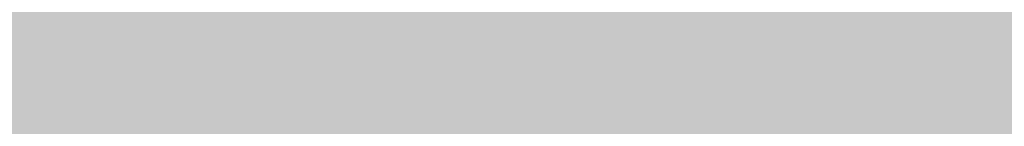
# Model space of a CAD drawing. Units: millimetres. Extents: x -22994 to 29398, y -19990 to 20176.
# Tile 77 of 135: x 226.355 to 227.437, y 84.615 to 84.732. Entities that reach past the tile are written whole.
import ezdxf
from ezdxf import colors
from ezdxf.entities.mleader import LeaderData, LeaderLine
from ezdxf.math import Vec2, Vec3

# ---------------------------------------------------------------- set-up
doc = ezdxf.new("R2010")
doc.units = ezdxf.units.MM
doc.header["$MEASUREMENT"] = 0
doc.layers.add('M-ANNO-TEXT', color=7, linetype='Continuous', lineweight=25)
doc.layers.add('M-DIMS', color=2, linetype='Continuous', lineweight=18)
doc.styles.get("Standard").update_dxf_attribs({"font": 'arial.ttf'})
doc.dimstyles.get("Standard").update_dxf_attribs({"dimtxt": 0.18, "dimasz": 10000, "dimexe": 0.18, "dimexo": 0.0625, "dimgap": 0.09, "dimtad": 0, "dimtih": 1, "dimtoh": 1, "dimdec": 0, "dimzin": 0, "dimdsep": 46, "dimtxsty": 'Standard', "dimcen": 0.09, "dimadec": 0, "dimazin": 0, "dimtfac": 1, "dimtdec": 0, "dimtofl": 0, "dimtmove": 0, "dimatfit": 3, "dimfxl": 1, "dimtolj": 1, "dimtzin": 0, "dimlwd": 30, "dimarcsym": 0})

# ---------------------------------------------------------------- blocks, each defined once
blk = doc.blocks.new('*D2')
at = {"layer": 'Defpoints', "color": 0, "transparency": 16777216}
for p in [(6.6773, 10.2713), (290.852, 10.2713), (290.852, -5.0787)]:
    blk.add_point(p, dxfattribs=at)
at = {"layer": 'M-DIMS', "color": 0, "lineweight": -2, "transparency": 16777216}
for p, q in [((6.6773, 10.2088), (6.6773, -5.2587)), ((290.852, 10.2088), (290.852, -5.2587))]:
    blk.add_line(p, q, dxfattribs=at)
at = {"layer": 'M-DIMS', "color": 0, "lineweight": 30, "transparency": 16777216}
for p, q in [((-9993.3227, -5.0787), (-19993.3227, -5.0787)), ((10290.852, -5.0787), (20290.852, -5.0787))]:
    blk.add_line(p, q, dxfattribs=at)
at = {"layer": 'M-DIMS', "color": 0, "transparency": 16777216}
for points in [[(-9993.3227, 1661.5879), (-9993.3227, -1671.7454), (6.6773, -5.0787)], [(10290.852, 1661.5879), (10290.852, -1671.7454), (290.852, -5.0787)]]:
    blk.add_solid(points, dxfattribs=at)
at = {"layer": 'M-DIMS', "color": 0, "transparency": 16777216, "insert": (148.7647, -5.0787), "char_height": 0.18, "attachment_point": 5}
blk.add_mtext('\\A1;284.2', dxfattribs=at)
blk = doc.blocks.new('*D3')
at = {"layer": 'Defpoints', "color": 0, "transparency": 16777216}
for p in [(110.2647, 204.1654), (110.2647, 176.3662), (95.8327, 127.967)]:
    blk.add_point(p, dxfattribs=at)
at = {"layer": 'M-DIMS', "color": 0, "lineweight": -2, "transparency": 16777216}
for p, q in [((95.8327, 128.0295), (95.8327, 204.3454)), ((110.2647, 176.4287), (110.2647, 204.3454))]:
    blk.add_line(p, q, dxfattribs=at)
at = {"layer": 'M-DIMS', "color": 0, "lineweight": 30, "transparency": 16777216}
for p, q in [((-9904.1673, 204.1654), (-19904.1673, 204.1654)), ((10110.2647, 204.1654), (20110.2647, 204.1654))]:
    blk.add_line(p, q, dxfattribs=at)
at = {"layer": 'M-DIMS', "color": 0, "transparency": 16777216}
for points in [[(-9904.1673, 1870.8321), (-9904.1673, -1462.5013), (95.8327, 204.1654)], [(10110.2647, 1870.8321), (10110.2647, -1462.5013), (110.2647, 204.1654)]]:
    blk.add_solid(points, dxfattribs=at)
at = {"layer": 'M-DIMS', "color": 0, "transparency": 16777216, "insert": (103.0487, 204.1654), "char_height": 0.18, "attachment_point": 5}
blk.add_mtext('\\A1;14.432', dxfattribs=at)
blk = doc.blocks.new('*D4')
at = {"layer": 'Defpoints', "color": 0, "transparency": 16777216}
for p in [(116.2647, 204.1654), (110.2647, 176.3662), (116.2647, 176.3662)]:
    blk.add_point(p, dxfattribs=at)
at = {"layer": 'M-DIMS', "color": 0, "lineweight": -2, "transparency": 16777216}
for p, q in [((110.2647, 176.4287), (110.2647, 204.3454)), ((116.2647, 176.4287), (116.2647, 204.3454))]:
    blk.add_line(p, q, dxfattribs=at)
at = {"layer": 'M-DIMS', "color": 0, "lineweight": 30, "transparency": 16777216}
for p, q in [((-9889.7353, 204.1654), (-19889.7353, 204.1654)), ((10116.2647, 204.1654), (20116.2647, 204.1654))]:
    blk.add_line(p, q, dxfattribs=at)
at = {"layer": 'M-DIMS', "color": 0, "transparency": 16777216}
for points in [[(-9889.7353, 1870.8321), (-9889.7353, -1462.5013), (110.2647, 204.1654)], [(10116.2647, 1870.8321), (10116.2647, -1462.5013), (116.2647, 204.1654)]]:
    blk.add_solid(points, dxfattribs=at)
at = {"layer": 'M-DIMS', "color": 0, "transparency": 16777216, "insert": (113.2647, 204.1654), "char_height": 0.18, "attachment_point": 5}
blk.add_mtext('\\A1;6', dxfattribs=at)
blk = doc.blocks.new('*D5')
at = {"layer": 'Defpoints', "color": 0, "transparency": 16777216}
for p in [(181.2647, 204.1654), (116.2647, 176.3662), (181.2647, 176.3662)]:
    blk.add_point(p, dxfattribs=at)
at = {"layer": 'M-DIMS', "color": 0, "lineweight": -2, "transparency": 16777216}
for p, q in [((116.2647, 176.4287), (116.2647, 204.3454)), ((181.2647, 176.4287), (181.2647, 204.3454))]:
    blk.add_line(p, q, dxfattribs=at)
at = {"layer": 'M-DIMS', "color": 0, "lineweight": 30, "transparency": 16777216}
for p, q in [((-9883.7353, 204.1654), (-19883.7353, 204.1654)), ((10181.2647, 204.1654), (20181.2647, 204.1654))]:
    blk.add_line(p, q, dxfattribs=at)
at = {"layer": 'M-DIMS', "color": 0, "transparency": 16777216}
for points in [[(-9883.7353, 1870.8321), (-9883.7353, -1462.5013), (116.2647, 204.1654)], [(10181.2647, 1870.8321), (10181.2647, -1462.5013), (181.2647, 204.1654)]]:
    blk.add_solid(points, dxfattribs=at)
at = {"layer": 'M-DIMS', "color": 0, "transparency": 16777216, "insert": (148.7647, 204.1654), "char_height": 0.18, "attachment_point": 5}
blk.add_mtext('\\A1;65', dxfattribs=at)
blk = doc.blocks.new('*D6')
at = {"layer": 'Defpoints', "color": 0, "transparency": 16777216}
for p in [(187.2647, 204.1654), (181.2647, 176.3662), (187.2647, 176.3662)]:
    blk.add_point(p, dxfattribs=at)
at = {"layer": 'M-DIMS', "color": 0, "lineweight": -2, "transparency": 16777216}
for p, q in [((181.2647, 176.4287), (181.2647, 204.3454)), ((187.2647, 176.4287), (187.2647, 204.3454))]:
    blk.add_line(p, q, dxfattribs=at)
at = {"layer": 'M-DIMS', "color": 0, "lineweight": 30, "transparency": 16777216}
for p, q in [((-9818.7353, 204.1654), (-19818.7353, 204.1654)), ((10187.2647, 204.1654), (20187.2647, 204.1654))]:
    blk.add_line(p, q, dxfattribs=at)
at = {"layer": 'M-DIMS', "color": 0, "transparency": 16777216}
for points in [[(-9818.7353, 1870.8321), (-9818.7353, -1462.5013), (181.2647, 204.1654)], [(10187.2647, 1870.8321), (10187.2647, -1462.5013), (187.2647, 204.1654)]]:
    blk.add_solid(points, dxfattribs=at)
at = {"layer": 'M-DIMS', "color": 0, "transparency": 16777216, "insert": (184.2647, 204.1654), "char_height": 0.18, "attachment_point": 5}
blk.add_mtext('\\A1;6', dxfattribs=at)
blk = doc.blocks.new('*D7')
at = {"layer": 'Defpoints', "color": 0, "transparency": 16777216}
for p in [(201.6967, 204.1654), (187.2647, 176.3662), (201.6967, 127.967)]:
    blk.add_point(p, dxfattribs=at)
at = {"layer": 'M-DIMS', "color": 0, "lineweight": -2, "transparency": 16777216}
for p, q in [((187.2647, 176.4287), (187.2647, 204.3454)), ((201.6967, 128.0295), (201.6967, 204.3454))]:
    blk.add_line(p, q, dxfattribs=at)
at = {"layer": 'M-DIMS', "color": 0, "lineweight": 30, "transparency": 16777216}
for p, q in [((-9812.7353, 204.1654), (-19812.7353, 204.1654)), ((10201.6967, 204.1654), (20201.6967, 204.1654))]:
    blk.add_line(p, q, dxfattribs=at)
at = {"layer": 'M-DIMS', "color": 0, "transparency": 16777216}
for points in [[(-9812.7353, 1870.8321), (-9812.7353, -1462.5013), (187.2647, 204.1654)], [(10201.6967, 1870.8321), (10201.6967, -1462.5013), (201.6967, 204.1654)]]:
    blk.add_solid(points, dxfattribs=at)
at = {"layer": 'M-DIMS', "color": 0, "transparency": 16777216, "insert": (194.4807, 204.1654), "char_height": 0.18, "attachment_point": 5}
blk.add_mtext('\\A1;14.432', dxfattribs=at)
blk = doc.blocks.new('*D8')
at = {"layer": 'Defpoints', "color": 0, "transparency": 16777216}
for p in [(227.6485, 204.1654), (227.6485, 146.7296), (201.6967, 127.967)]:
    blk.add_point(p, dxfattribs=at)
at = {"layer": 'M-DIMS', "color": 0, "lineweight": -2, "transparency": 16777216}
for p, q in [((201.6967, 128.0295), (201.6967, 204.3454)), ((227.6485, 146.7921), (227.6485, 204.3454))]:
    blk.add_line(p, q, dxfattribs=at)
at = {"layer": 'M-DIMS', "color": 0, "lineweight": 30, "transparency": 16777216}
for p, q in [((-9798.3033, 204.1654), (-19798.3033, 204.1654)), ((10227.6485, 204.1654), (20227.6485, 204.1654))]:
    blk.add_line(p, q, dxfattribs=at)
at = {"layer": 'M-DIMS', "color": 0, "transparency": 16777216}
for points in [[(-9798.3033, 1870.8321), (-9798.3033, -1462.5013), (201.6967, 204.1654)], [(10227.6485, 1870.8321), (10227.6485, -1462.5013), (227.6485, 204.1654)]]:
    blk.add_solid(points, dxfattribs=at)
at = {"layer": 'M-DIMS', "color": 0, "transparency": 16777216, "insert": (214.6726, 204.1654), "char_height": 0.18, "attachment_point": 5}
blk.add_mtext('\\A1;25.95', dxfattribs=at)
blk = doc.blocks.new('*D9')
at = {"layer": 'Defpoints', "color": 0, "transparency": 16777216}
for p in [(187.2647, 176.3662), (306.202, 176.3662), (290.852, 10.2713)]:
    blk.add_point(p, dxfattribs=at)
at = {"layer": 'M-DIMS', "color": 0, "lineweight": 30, "transparency": 16777216}
for p, q in [((306.202, 10176.3662), (306.202, 20176.3662)), ((306.202, -9989.7287), (306.202, -19989.7287))]:
    blk.add_line(p, q, dxfattribs=at)
at = {"layer": 'M-DIMS', "color": 0, "lineweight": -2, "transparency": 16777216}
for p, q in [((187.3272, 176.3662), (306.382, 176.3662)), ((290.9145, 10.2713), (306.382, 10.2713))]:
    blk.add_line(p, q, dxfattribs=at)
at = {"layer": 'M-DIMS', "color": 0, "transparency": 16777216}
for points in [[(-1360.4646, 10176.3662), (1972.8687, 10176.3662), (306.202, 176.3662)], [(-1360.4646, -9989.7287), (1972.8687, -9989.7287), (306.202, 10.2713)]]:
    blk.add_solid(points, dxfattribs=at)
at = {"layer": 'M-DIMS', "color": 0, "transparency": 16777216, "insert": (306.202, 93.3187), "char_height": 0.18, "attachment_point": 5}
blk.add_mtext('\\A1;166.1', dxfattribs=at)
blk = doc.blocks.new('*D10')
at = {"layer": 'Defpoints', "color": 0, "transparency": 16777216}
for p in [(125.6498, 136.0713), (133.3459, 136.0713), (133.3459, -5.0787)]:
    blk.add_point(p, dxfattribs=at)
at = {"layer": 'M-DIMS', "color": 0, "lineweight": -2, "transparency": 16777216}
for p, q in [((125.6498, 136.0088), (125.6498, -5.2587)), ((133.3459, 136.0088), (133.3459, -5.2587))]:
    blk.add_line(p, q, dxfattribs=at)
at = {"layer": 'M-DIMS', "color": 0, "lineweight": 30, "transparency": 16777216}
for p, q in [((-9874.3502, -5.0787), (-19874.3502, -5.0787)), ((10133.3459, -5.0787), (20133.3459, -5.0787))]:
    blk.add_line(p, q, dxfattribs=at)
at = {"layer": 'M-DIMS', "color": 0, "transparency": 16777216}
for points in [[(-9874.3502, 1661.5879), (-9874.3502, -1671.7454), (125.6498, -5.0787)], [(10133.3459, 1661.5879), (10133.3459, -1671.7454), (133.3459, -5.0787)]]:
    blk.add_solid(points, dxfattribs=at)
at = {"layer": 'M-DIMS', "color": 0, "transparency": 16777216, "insert": (129.4978, -5.0787), "char_height": 0.18, "attachment_point": 5}
blk.add_mtext('\\A1;7.696', dxfattribs=at)
blk = doc.blocks.new('*D11')
at = {"layer": 'Defpoints', "color": 0, "transparency": 16777216}
for p in [(133.3459, 136.0713), (135.6498, 136.0713), (135.6498, -5.0787)]:
    blk.add_point(p, dxfattribs=at)
at = {"layer": 'M-DIMS', "color": 0, "lineweight": -2, "transparency": 16777216}
for p, q in [((133.3459, 136.0088), (133.3459, -5.2587)), ((135.6498, 136.0088), (135.6498, -5.2587))]:
    blk.add_line(p, q, dxfattribs=at)
at = {"layer": 'M-DIMS', "color": 0, "lineweight": 30, "transparency": 16777216}
for p, q in [((-9866.6541, -5.0787), (-19866.6541, -5.0787)), ((10135.6498, -5.0787), (20135.6498, -5.0787))]:
    blk.add_line(p, q, dxfattribs=at)
at = {"layer": 'M-DIMS', "color": 0, "transparency": 16777216}
for points in [[(-9866.6541, 1661.5879), (-9866.6541, -1671.7454), (133.3459, -5.0787)], [(10135.6498, 1661.5879), (10135.6498, -1671.7454), (135.6498, -5.0787)]]:
    blk.add_solid(points, dxfattribs=at)
at = {"layer": 'M-DIMS', "color": 0, "transparency": 16777216, "insert": (134.4978, -5.0787), "char_height": 0.18, "attachment_point": 5}
blk.add_mtext('\\A1;2.304', dxfattribs=at)
blk = doc.blocks.new('*D12')
at = {"layer": 'Defpoints', "color": 0, "transparency": 16777216}
for p in [(135.6498, 136.0713), (145.6498, 136.0713), (145.6498, -5.0787)]:
    blk.add_point(p, dxfattribs=at)
at = {"layer": 'M-DIMS', "color": 0, "lineweight": -2, "transparency": 16777216}
for p, q in [((135.6498, 136.0088), (135.6498, -5.2587)), ((145.6498, 136.0088), (145.6498, -5.2587))]:
    blk.add_line(p, q, dxfattribs=at)
at = {"layer": 'M-DIMS', "color": 0, "lineweight": 30, "transparency": 16777216}
for p, q in [((-9864.3502, -5.0787), (-19864.3502, -5.0787)), ((10145.6498, -5.0787), (20145.6498, -5.0787))]:
    blk.add_line(p, q, dxfattribs=at)
at = {"layer": 'M-DIMS', "color": 0, "transparency": 16777216}
for points in [[(-9864.3502, 1661.5879), (-9864.3502, -1671.7454), (135.6498, -5.0787)], [(10145.6498, 1661.5879), (10145.6498, -1671.7454), (145.6498, -5.0787)]]:
    blk.add_solid(points, dxfattribs=at)
at = {"layer": 'M-DIMS', "color": 0, "transparency": 16777216, "insert": (140.6498, -5.0787), "char_height": 0.18, "attachment_point": 5}
blk.add_mtext('\\A1;10', dxfattribs=at)
blk = doc.blocks.new('*D13')
at = {"layer": 'Defpoints', "color": 0, "transparency": 16777216}
for p in [(145.6498, 136.0713), (155.6498, 136.0713), (155.6498, -5.0787)]:
    blk.add_point(p, dxfattribs=at)
at = {"layer": 'M-DIMS', "color": 0, "lineweight": -2, "transparency": 16777216}
for p, q in [((145.6498, 136.0088), (145.6498, -5.2587)), ((155.6498, 136.0088), (155.6498, -5.2587))]:
    blk.add_line(p, q, dxfattribs=at)
at = {"layer": 'M-DIMS', "color": 0, "lineweight": 30, "transparency": 16777216}
for p, q in [((-9854.3502, -5.0787), (-19854.3502, -5.0787)), ((10155.6498, -5.0787), (20155.6498, -5.0787))]:
    blk.add_line(p, q, dxfattribs=at)
at = {"layer": 'M-DIMS', "color": 0, "transparency": 16777216}
for points in [[(-9854.3502, 1661.5879), (-9854.3502, -1671.7454), (145.6498, -5.0787)], [(10155.6498, 1661.5879), (10155.6498, -1671.7454), (155.6498, -5.0787)]]:
    blk.add_solid(points, dxfattribs=at)
at = {"layer": 'M-DIMS', "color": 0, "transparency": 16777216, "insert": (150.6498, -5.0787), "char_height": 0.18, "attachment_point": 5}
blk.add_mtext('\\A1;10', dxfattribs=at)
blk = doc.blocks.new('*D14')
at = {"layer": 'Defpoints', "color": 0, "transparency": 16777216}
for p in [(155.6498, 136.0713), (165.6498, 136.0713), (165.6498, -5.0787)]:
    blk.add_point(p, dxfattribs=at)
at = {"layer": 'M-DIMS', "color": 0, "lineweight": -2, "transparency": 16777216}
for p, q in [((155.6498, 136.0088), (155.6498, -5.2587)), ((165.6498, 136.0088), (165.6498, -5.2587))]:
    blk.add_line(p, q, dxfattribs=at)
at = {"layer": 'M-DIMS', "color": 0, "lineweight": 30, "transparency": 16777216}
for p, q in [((-9844.3502, -5.0787), (-19844.3502, -5.0787)), ((10165.6498, -5.0787), (20165.6498, -5.0787))]:
    blk.add_line(p, q, dxfattribs=at)
at = {"layer": 'M-DIMS', "color": 0, "transparency": 16777216}
for points in [[(-9844.3502, 1661.5879), (-9844.3502, -1671.7454), (155.6498, -5.0787)], [(10165.6498, 1661.5879), (10165.6498, -1671.7454), (165.6498, -5.0787)]]:
    blk.add_solid(points, dxfattribs=at)
at = {"layer": 'M-DIMS', "color": 0, "transparency": 16777216, "insert": (160.6498, -5.0787), "char_height": 0.18, "attachment_point": 5}
blk.add_mtext('\\A1;10', dxfattribs=at)
blk = doc.blocks.new('*D15')
at = {"layer": 'Defpoints', "color": 0, "transparency": 16777216}
for p in [(173.3459, 154.788), (173.3459, 136.0713), (306.202, 136.0713)]:
    blk.add_point(p, dxfattribs=at)
at = {"layer": 'M-DIMS', "color": 0, "lineweight": 30, "transparency": 16777216}
for p, q in [((306.202, 10154.788), (306.202, 20154.788)), ((306.202, -9863.9287), (306.202, -19863.9287))]:
    blk.add_line(p, q, dxfattribs=at)
at = {"layer": 'M-DIMS', "color": 0, "lineweight": -2, "transparency": 16777216}
for p, q in [((173.4084, 154.788), (306.382, 154.788)), ((173.4084, 136.0713), (306.382, 136.0713))]:
    blk.add_line(p, q, dxfattribs=at)
at = {"layer": 'M-DIMS', "color": 0, "transparency": 16777216}
for points in [[(-1360.4646, 10154.788), (1972.8687, 10154.788), (306.202, 154.788)], [(-1360.4646, -9863.9287), (1972.8687, -9863.9287), (306.202, 136.0713)]]:
    blk.add_solid(points, dxfattribs=at)
at = {"layer": 'M-DIMS', "color": 0, "transparency": 16777216, "insert": (306.202, 145.4297), "char_height": 0.18, "attachment_point": 5}
blk.add_mtext('\\A1;18.717', dxfattribs=at)
blk = doc.blocks.new('*D16')
at = {"layer": 'Defpoints', "color": 0, "transparency": 16777216}
for p in [(120.1702, 204.1654), (110.4658, 48.0349), (120.1702, 48.0349)]:
    blk.add_point(p, dxfattribs=at)
at = {"layer": 'M-DIMS', "color": 0, "lineweight": -2, "transparency": 16777216}
for p, q in [((110.4658, 48.0974), (110.4658, 204.3454)), ((120.1702, 48.0974), (120.1702, 204.3454))]:
    blk.add_line(p, q, dxfattribs=at)
at = {"layer": 'M-DIMS', "color": 0, "lineweight": 30, "transparency": 16777216}
for p, q in [((-9889.5342, 204.1654), (-19889.5342, 204.1654)), ((10120.1702, 204.1654), (20120.1702, 204.1654))]:
    blk.add_line(p, q, dxfattribs=at)
at = {"layer": 'M-DIMS', "color": 0, "transparency": 16777216}
for points in [[(-9889.5342, 1870.8321), (-9889.5342, -1462.5013), (110.4658, 204.1654)], [(10120.1702, 1870.8321), (10120.1702, -1462.5013), (120.1702, 204.1654)]]:
    blk.add_solid(points, dxfattribs=at)
at = {"layer": 'M-DIMS', "color": 0, "transparency": 16777216, "insert": (115.318, 204.1654), "char_height": 0.18, "attachment_point": 5}
blk.add_mtext('\\A1;9.704', dxfattribs=at)
blk = doc.blocks.new('*D17')
at = {"layer": 'Defpoints', "color": 0, "transparency": 16777216}
for p in [(126.1702, 204.1654), (120.1702, 48.0349), (126.1702, 48.0349)]:
    blk.add_point(p, dxfattribs=at)
at = {"layer": 'M-DIMS', "color": 0, "lineweight": -2, "transparency": 16777216}
for p, q in [((120.1702, 48.0974), (120.1702, 204.3454)), ((126.1702, 48.0974), (126.1702, 204.3454))]:
    blk.add_line(p, q, dxfattribs=at)
at = {"layer": 'M-DIMS', "color": 0, "lineweight": 30, "transparency": 16777216}
for p, q in [((-9879.8298, 204.1654), (-19879.8298, 204.1654)), ((10126.1702, 204.1654), (20126.1702, 204.1654))]:
    blk.add_line(p, q, dxfattribs=at)
at = {"layer": 'M-DIMS', "color": 0, "transparency": 16777216}
for points in [[(-9879.8298, 1870.8321), (-9879.8298, -1462.5013), (120.1702, 204.1654)], [(10126.1702, 1870.8321), (10126.1702, -1462.5013), (126.1702, 204.1654)]]:
    blk.add_solid(points, dxfattribs=at)
at = {"layer": 'M-DIMS', "color": 0, "transparency": 16777216, "insert": (123.1702, 204.1654), "char_height": 0.18, "attachment_point": 5}
blk.add_mtext('\\A1;6', dxfattribs=at)
blk = doc.blocks.new('*D18')
at = {"layer": 'Defpoints', "color": 0, "transparency": 16777216}
for p in [(132.1702, 204.1654), (126.1702, 48.0349), (132.1702, 48.0349)]:
    blk.add_point(p, dxfattribs=at)
at = {"layer": 'M-DIMS', "color": 0, "lineweight": -2, "transparency": 16777216}
for p, q in [((126.1702, 48.0974), (126.1702, 204.3454)), ((132.1702, 48.0974), (132.1702, 204.3454))]:
    blk.add_line(p, q, dxfattribs=at)
at = {"layer": 'M-DIMS', "color": 0, "lineweight": 30, "transparency": 16777216}
for p, q in [((-9873.8298, 204.1654), (-19873.8298, 204.1654)), ((10132.1702, 204.1654), (20132.1702, 204.1654))]:
    blk.add_line(p, q, dxfattribs=at)
at = {"layer": 'M-DIMS', "color": 0, "transparency": 16777216}
for points in [[(-9873.8298, 1870.8321), (-9873.8298, -1462.5013), (126.1702, 204.1654)], [(10132.1702, 1870.8321), (10132.1702, -1462.5013), (132.1702, 204.1654)]]:
    blk.add_solid(points, dxfattribs=at)
at = {"layer": 'M-DIMS', "color": 0, "transparency": 16777216, "insert": (129.1702, 204.1654), "char_height": 0.18, "attachment_point": 5}
blk.add_mtext('\\A1;6', dxfattribs=at)
blk = doc.blocks.new('*D19')
at = {"layer": 'Defpoints', "color": 0, "transparency": 16777216}
for p in [(138.1702, 204.1654), (132.1702, 48.0349), (138.1702, 48.0349)]:
    blk.add_point(p, dxfattribs=at)
at = {"layer": 'M-DIMS', "color": 0, "lineweight": -2, "transparency": 16777216}
for p, q in [((132.1702, 48.0974), (132.1702, 204.3454)), ((138.1702, 48.0974), (138.1702, 204.3454))]:
    blk.add_line(p, q, dxfattribs=at)
at = {"layer": 'M-DIMS', "color": 0, "lineweight": 30, "transparency": 16777216}
for p, q in [((-9867.8298, 204.1654), (-19867.8298, 204.1654)), ((10138.1702, 204.1654), (20138.1702, 204.1654))]:
    blk.add_line(p, q, dxfattribs=at)
at = {"layer": 'M-DIMS', "color": 0, "transparency": 16777216}
for points in [[(-9867.8298, 1870.8321), (-9867.8298, -1462.5013), (132.1702, 204.1654)], [(10138.1702, 1870.8321), (10138.1702, -1462.5013), (138.1702, 204.1654)]]:
    blk.add_solid(points, dxfattribs=at)
at = {"layer": 'M-DIMS', "color": 0, "transparency": 16777216, "insert": (135.1702, 204.1654), "char_height": 0.18, "attachment_point": 5}
blk.add_mtext('\\A1;6', dxfattribs=at)
blk = doc.blocks.new('*D20')
at = {"layer": 'Defpoints', "color": 0, "transparency": 16777216}
for p in [(144.1702, 204.1654), (138.1702, 48.0349), (144.1702, 48.0349)]:
    blk.add_point(p, dxfattribs=at)
at = {"layer": 'M-DIMS', "color": 0, "lineweight": -2, "transparency": 16777216}
for p, q in [((138.1702, 48.0974), (138.1702, 204.3454)), ((144.1702, 48.0974), (144.1702, 204.3454))]:
    blk.add_line(p, q, dxfattribs=at)
at = {"layer": 'M-DIMS', "color": 0, "lineweight": 30, "transparency": 16777216}
for p, q in [((-9861.8298, 204.1654), (-19861.8298, 204.1654)), ((10144.1702, 204.1654), (20144.1702, 204.1654))]:
    blk.add_line(p, q, dxfattribs=at)
at = {"layer": 'M-DIMS', "color": 0, "transparency": 16777216}
for points in [[(-9861.8298, 1870.8321), (-9861.8298, -1462.5013), (138.1702, 204.1654)], [(10144.1702, 1870.8321), (10144.1702, -1462.5013), (144.1702, 204.1654)]]:
    blk.add_solid(points, dxfattribs=at)
at = {"layer": 'M-DIMS', "color": 0, "transparency": 16777216, "insert": (141.1702, 204.1654), "char_height": 0.18, "attachment_point": 5}
blk.add_mtext('\\A1;6', dxfattribs=at)
blk = doc.blocks.new('*D21')
at = {"layer": 'Defpoints', "color": 0, "transparency": 16777216}
for p in [(149.1157, 204.1654), (144.1702, 48.0349), (149.1157, 48.0349)]:
    blk.add_point(p, dxfattribs=at)
at = {"layer": 'M-DIMS', "color": 0, "lineweight": -2, "transparency": 16777216}
for p, q in [((144.1702, 48.0974), (144.1702, 204.3454)), ((149.1157, 48.0974), (149.1157, 204.3454))]:
    blk.add_line(p, q, dxfattribs=at)
at = {"layer": 'M-DIMS', "color": 0, "lineweight": 30, "transparency": 16777216}
for p, q in [((-9855.8298, 204.1654), (-19855.8298, 204.1654)), ((10149.1157, 204.1654), (20149.1157, 204.1654))]:
    blk.add_line(p, q, dxfattribs=at)
at = {"layer": 'M-DIMS', "color": 0, "transparency": 16777216}
for points in [[(-9855.8298, 1870.8321), (-9855.8298, -1462.5013), (144.1702, 204.1654)], [(10149.1157, 1870.8321), (10149.1157, -1462.5013), (149.1157, 204.1654)]]:
    blk.add_solid(points, dxfattribs=at)
at = {"layer": 'M-DIMS', "color": 0, "transparency": 16777216, "insert": (146.6429, 204.1654), "char_height": 0.18, "attachment_point": 5}
blk.add_mtext('\\A1;4.945', dxfattribs=at)
blk = doc.blocks.new('*D22')
at = {"layer": 'Defpoints', "color": 0, "transparency": 16777216}
for p in [(149.1157, 30.9895), (155.1157, 30.9895), (155.1157, -5.0787)]:
    blk.add_point(p, dxfattribs=at)
at = {"layer": 'M-DIMS', "color": 0, "lineweight": -2, "transparency": 16777216}
for p, q in [((149.1157, 30.927), (149.1157, -5.2587)), ((155.1157, 30.927), (155.1157, -5.2587))]:
    blk.add_line(p, q, dxfattribs=at)
at = {"layer": 'M-DIMS', "color": 0, "lineweight": 30, "transparency": 16777216}
for p, q in [((-9850.8843, -5.0787), (-19850.8843, -5.0787)), ((10155.1157, -5.0787), (20155.1157, -5.0787))]:
    blk.add_line(p, q, dxfattribs=at)
at = {"layer": 'M-DIMS', "color": 0, "transparency": 16777216}
for points in [[(-9850.8843, 1661.5879), (-9850.8843, -1671.7454), (149.1157, -5.0787)], [(10155.1157, 1661.5879), (10155.1157, -1671.7454), (155.1157, -5.0787)]]:
    blk.add_solid(points, dxfattribs=at)
at = {"layer": 'M-DIMS', "color": 0, "transparency": 16777216, "insert": (152.1157, -5.0787), "char_height": 0.18, "attachment_point": 5}
blk.add_mtext('\\A1;6', dxfattribs=at)
blk = doc.blocks.new('*D23')
at = {"layer": 'Defpoints', "color": 0, "transparency": 16777216}
for p in [(155.1157, 30.9895), (161.1157, 30.9895), (161.1157, -5.0787)]:
    blk.add_point(p, dxfattribs=at)
at = {"layer": 'M-DIMS', "color": 0, "lineweight": -2, "transparency": 16777216}
for p, q in [((155.1157, 30.927), (155.1157, -5.2587)), ((161.1157, 30.927), (161.1157, -5.2587))]:
    blk.add_line(p, q, dxfattribs=at)
at = {"layer": 'M-DIMS', "color": 0, "lineweight": 30, "transparency": 16777216}
for p, q in [((-9844.8843, -5.0787), (-19844.8843, -5.0787)), ((10161.1157, -5.0787), (20161.1157, -5.0787))]:
    blk.add_line(p, q, dxfattribs=at)
at = {"layer": 'M-DIMS', "color": 0, "transparency": 16777216}
for points in [[(-9844.8843, 1661.5879), (-9844.8843, -1671.7454), (155.1157, -5.0787)], [(10161.1157, 1661.5879), (10161.1157, -1671.7454), (161.1157, -5.0787)]]:
    blk.add_solid(points, dxfattribs=at)
at = {"layer": 'M-DIMS', "color": 0, "transparency": 16777216, "insert": (158.1157, -5.0787), "char_height": 0.18, "attachment_point": 5}
blk.add_mtext('\\A1;6', dxfattribs=at)
blk = doc.blocks.new('*D24')
at = {"layer": 'Defpoints', "color": 0, "transparency": 16777216}
for p in [(161.1157, 30.9895), (166.4387, 30.9895), (166.4387, -5.0787)]:
    blk.add_point(p, dxfattribs=at)
at = {"layer": 'M-DIMS', "color": 0, "lineweight": -2, "transparency": 16777216}
for p, q in [((161.1157, 30.927), (161.1157, -5.2587)), ((166.4387, 30.927), (166.4387, -5.2587))]:
    blk.add_line(p, q, dxfattribs=at)
at = {"layer": 'M-DIMS', "color": 0, "lineweight": 30, "transparency": 16777216}
for p, q in [((-9838.8843, -5.0787), (-19838.8843, -5.0787)), ((10166.4387, -5.0787), (20166.4387, -5.0787))]:
    blk.add_line(p, q, dxfattribs=at)
at = {"layer": 'M-DIMS', "color": 0, "transparency": 16777216}
for points in [[(-9838.8843, 1661.5879), (-9838.8843, -1671.7454), (161.1157, -5.0787)], [(10166.4387, 1661.5879), (10166.4387, -1671.7454), (166.4387, -5.0787)]]:
    blk.add_solid(points, dxfattribs=at)
at = {"layer": 'M-DIMS', "color": 0, "transparency": 16777216, "insert": (163.7772, -5.0787), "char_height": 0.18, "attachment_point": 5}
blk.add_mtext('\\A1;5.323', dxfattribs=at)
blk = doc.blocks.new('*D25')
at = {"layer": 'Defpoints', "color": 0, "transparency": 16777216}
for p in [(166.4387, 30.9895), (172.4387, 30.9895), (172.4387, -5.0787)]:
    blk.add_point(p, dxfattribs=at)
at = {"layer": 'M-DIMS', "color": 0, "lineweight": -2, "transparency": 16777216}
for p, q in [((166.4387, 30.927), (166.4387, -5.2587)), ((172.4387, 30.927), (172.4387, -5.2587))]:
    blk.add_line(p, q, dxfattribs=at)
at = {"layer": 'M-DIMS', "color": 0, "lineweight": 30, "transparency": 16777216}
for p, q in [((-9833.5613, -5.0787), (-19833.5613, -5.0787)), ((10172.4387, -5.0787), (20172.4387, -5.0787))]:
    blk.add_line(p, q, dxfattribs=at)
at = {"layer": 'M-DIMS', "color": 0, "transparency": 16777216}
for points in [[(-9833.5613, 1661.5879), (-9833.5613, -1671.7454), (166.4387, -5.0787)], [(10172.4387, 1661.5879), (10172.4387, -1671.7454), (172.4387, -5.0787)]]:
    blk.add_solid(points, dxfattribs=at)
at = {"layer": 'M-DIMS', "color": 0, "transparency": 16777216, "insert": (169.4387, -5.0787), "char_height": 0.18, "attachment_point": 5}
blk.add_mtext('\\A1;6', dxfattribs=at)
blk = doc.blocks.new('*D26')
at = {"layer": 'Defpoints', "color": 0, "transparency": 16777216}
for p in [(172.4387, 30.9895), (178.4387, 30.9895), (178.4387, -5.0787)]:
    blk.add_point(p, dxfattribs=at)
at = {"layer": 'M-DIMS', "color": 0, "lineweight": -2, "transparency": 16777216}
for p, q in [((172.4387, 30.927), (172.4387, -5.2587)), ((178.4387, 30.927), (178.4387, -5.2587))]:
    blk.add_line(p, q, dxfattribs=at)
at = {"layer": 'M-DIMS', "color": 0, "lineweight": 30, "transparency": 16777216}
for p, q in [((-9827.5613, -5.0787), (-19827.5613, -5.0787)), ((10178.4387, -5.0787), (20178.4387, -5.0787))]:
    blk.add_line(p, q, dxfattribs=at)
at = {"layer": 'M-DIMS', "color": 0, "transparency": 16777216}
for points in [[(-9827.5613, 1661.5879), (-9827.5613, -1671.7454), (172.4387, -5.0787)], [(10178.4387, 1661.5879), (10178.4387, -1671.7454), (178.4387, -5.0787)]]:
    blk.add_solid(points, dxfattribs=at)
at = {"layer": 'M-DIMS', "color": 0, "transparency": 16777216, "insert": (175.4387, -5.0787), "char_height": 0.18, "attachment_point": 5}
blk.add_mtext('\\A1;6', dxfattribs=at)
blk = doc.blocks.new('*D27')
at = {"layer": 'Defpoints', "color": 0, "transparency": 16777216}
for p in [(178.4387, 30.9895), (188.1175, 30.9895), (188.1175, -5.0787)]:
    blk.add_point(p, dxfattribs=at)
at = {"layer": 'M-DIMS', "color": 0, "lineweight": -2, "transparency": 16777216}
for p, q in [((178.4387, 30.927), (178.4387, -5.2587)), ((188.1175, 30.927), (188.1175, -5.2587))]:
    blk.add_line(p, q, dxfattribs=at)
at = {"layer": 'M-DIMS', "color": 0, "lineweight": 30, "transparency": 16777216}
for p, q in [((-9821.5613, -5.0787), (-19821.5613, -5.0787)), ((10188.1175, -5.0787), (20188.1175, -5.0787))]:
    blk.add_line(p, q, dxfattribs=at)
at = {"layer": 'M-DIMS', "color": 0, "transparency": 16777216}
for points in [[(-9821.5613, 1661.5879), (-9821.5613, -1671.7454), (178.4387, -5.0787)], [(10188.1175, 1661.5879), (10188.1175, -1671.7454), (188.1175, -5.0787)]]:
    blk.add_solid(points, dxfattribs=at)
at = {"layer": 'M-DIMS', "color": 0, "transparency": 16777216, "insert": (183.2781, -5.0787), "char_height": 0.18, "attachment_point": 5}
blk.add_mtext('\\A1;9.679', dxfattribs=at)
blk = doc.blocks.new('*D28')
at = {"layer": 'Defpoints', "color": 0, "transparency": 16777216}
for p in [(188.1175, 48.0349), (306.202, 48.0349), (188.1175, 30.9895)]:
    blk.add_point(p, dxfattribs=at)
at = {"layer": 'M-DIMS', "color": 0, "lineweight": 30, "transparency": 16777216}
for p, q in [((306.202, 10048.0349), (306.202, 20048.0349)), ((306.202, -9969.0105), (306.202, -19969.0105))]:
    blk.add_line(p, q, dxfattribs=at)
at = {"layer": 'M-DIMS', "color": 0, "lineweight": -2, "transparency": 16777216}
for p, q in [((188.18, 48.0349), (306.382, 48.0349)), ((188.18, 30.9895), (306.382, 30.9895))]:
    blk.add_line(p, q, dxfattribs=at)
at = {"layer": 'M-DIMS', "color": 0, "transparency": 16777216}
for points in [[(-1360.4646, 10048.0349), (1972.8687, 10048.0349), (306.202, 48.0349)], [(-1360.4646, -9969.0105), (1972.8687, -9969.0105), (306.202, 30.9895)]]:
    blk.add_solid(points, dxfattribs=at)
at = {"layer": 'M-DIMS', "color": 0, "transparency": 16777216, "insert": (306.202, 39.5122), "char_height": 0.18, "attachment_point": 5}
blk.add_mtext('\\A1;17.045', dxfattribs=at)
blk = doc.blocks.new('*D29')
at = {"layer": 'Defpoints', "color": 0, "transparency": 16777216}
for p in [(36.8006, 80.045), (64.0296, 80.045)]:
    blk.add_point(p, dxfattribs=at)
at = {"layer": 'M-DIMS', "color": 0, "lineweight": -2, "transparency": 16777216}
for p, q in [((50.4151, 79.955), (50.4151, 80.135)), ((50.3251, 80.045), (50.5051, 80.045))]:
    blk.add_line(p, q, dxfattribs=at)
at = {"layer": 'M-DIMS', "color": 0, "lineweight": 30, "transparency": 16777216}
blk.add_line((20064.0296, 80.0303), (10064.0296, 80.0377), dxfattribs=at)
at = {"layer": 'M-DIMS', "color": 0, "transparency": 16777216}
blk.add_solid([(10064.0309, 1746.7043), (10064.0284, -1586.629), (64.0296, 80.045)], dxfattribs=at)
at = {"layer": 'M-DIMS', "color": 0, "transparency": 16777216, "insert": (20064.5213, 80.0303), "char_height": 0.18, "attachment_point": 5}
blk.add_mtext('\\A1;∅27.23', dxfattribs=at)
blk = doc.blocks.new('*D30')
at = {"layer": 'Defpoints', "color": 0, "transparency": 16777216}
for p in [(216.3148, 146.7291), (238.9821, 146.73)]:
    blk.add_point(p, dxfattribs=at)
at = {"layer": 'M-DIMS', "color": 0, "lineweight": 30, "transparency": 16777216}
blk.add_line((20238.9821, 147.4959), (10238.9821, 147.1129), dxfattribs=at)
at = {"layer": 'M-DIMS', "color": 0, "lineweight": -2, "transparency": 16777216}
for p, q in [((227.6485, 146.6396), (227.6485, 146.8196)), ((227.5585, 146.7296), (227.7385, 146.7296))]:
    blk.add_line(p, q, dxfattribs=at)
at = {"layer": 'M-DIMS', "color": 0, "transparency": 16777216}
blk.add_solid([(10238.9183, 1813.7796), (10239.0459, -1519.5537), (238.9821, 146.73)], dxfattribs=at)
at = {"layer": 'M-DIMS', "color": 0, "transparency": 16777216, "insert": (20239.5436, 147.4959), "char_height": 0.18, "attachment_point": 5}
blk.add_mtext('\\A1;∅22.667', dxfattribs=at)
blk = doc.blocks.new('*D31')
at = {"layer": 'Defpoints', "color": 0, "transparency": 16777216}
for p in [(223.1641, 146.7291), (232.1328, 146.73)]:
    blk.add_point(p, dxfattribs=at)
at = {"layer": 'M-DIMS', "color": 0, "lineweight": 30, "transparency": 16777216}
blk.add_line((20232.1327, 148.6656), (10232.1328, 147.6978), dxfattribs=at)
at = {"layer": 'M-DIMS', "color": 0, "lineweight": -2, "transparency": 16777216}
for p, q in [((227.6485, 146.6396), (227.6485, 146.8196)), ((227.5585, 146.7296), (227.7385, 146.7296))]:
    blk.add_line(p, q, dxfattribs=at)
at = {"layer": 'M-DIMS', "color": 0, "transparency": 16777216}
blk.add_solid([(10231.9715, 1814.3645), (10232.2941, -1518.9688), (232.1328, 146.73)], dxfattribs=at)
at = {"layer": 'M-DIMS', "color": 0, "transparency": 16777216, "insert": (20232.6245, 148.6656), "char_height": 0.18, "attachment_point": 5}
blk.add_mtext('\\A1;∅8.969', dxfattribs=at)
blk = doc.blocks.new('*D36')
at = {"layer": 'Defpoints', "color": 0, "transparency": 16777216}
for p in [(46.39, 31.3035), (46.3875, 26.5934)]:
    blk.add_point(p, dxfattribs=at)
at = {"layer": 'M-DIMS', "color": 0, "lineweight": 30, "transparency": 16777216}
for p, q in [((57.1499, 20031.3006), (51.77, 10031.302)), ((10057.1499, 20031.3006), (57.1499, 20031.3006))]:
    blk.add_line(p, q, dxfattribs=at)
at = {"layer": 'M-DIMS', "color": 0, "lineweight": -2, "transparency": 16777216}
for p, q in [((46.3887, 28.8585), (46.3887, 29.0385)), ((46.2987, 28.9485), (46.4787, 28.9485))]:
    blk.add_line(p, q, dxfattribs=at)
at = {"layer": 'M-DIMS', "color": 0, "transparency": 16777216}
blk.add_solid([(-1614.8965, 10032.1987), (1718.4364, 10030.4054), (46.39, 31.3035)], dxfattribs=at)
at = {"layer": 'M-DIMS', "color": 0, "transparency": 16777216, "insert": (10057.5542, 20031.3006), "char_height": 0.18, "attachment_point": 5}
blk.add_mtext('\\A1;∅4.71', dxfattribs=at)
blk = doc.blocks.new('*D37')
at = {"layer": 'Defpoints', "color": 0, "transparency": 16777216}
for p in [(54.8343, 118.6145), (59.4936, 118.614)]:
    blk.add_point(p, dxfattribs=at)
at = {"layer": 'M-DIMS', "color": 0, "lineweight": -2, "transparency": 16777216}
for p, q in [((57.1639, 118.5243), (57.1639, 118.7043)), ((57.0739, 118.6143), (57.2539, 118.6143))]:
    blk.add_line(p, q, dxfattribs=at)
at = {"layer": 'M-DIMS', "color": 0, "lineweight": 30, "transparency": 16777216}
blk.add_line((20059.4934, 116.2531), (10059.4935, 117.4336), dxfattribs=at)
at = {"layer": 'M-DIMS', "color": 0, "transparency": 16777216}
blk.add_solid([(10059.6902, 1784.1002), (10059.2968, -1549.2331), (59.4936, 118.614)], dxfattribs=at)
at = {"layer": 'M-DIMS', "color": 0, "transparency": 16777216, "insert": (20059.9852, 116.2531), "char_height": 0.18, "attachment_point": 5}
blk.add_mtext('\\A1;∅4.659', dxfattribs=at)

msp = doc.modelspace()

# ---------------------------------------------------------------- dimensions: what is measured, and where the dimension line sits
at = {"layer": 'M-DIMS'}
for base, p1, p2, override, picture, middle in [((306.202, 176.3662), (290.852, 10.2713), (187.2647, 176.3662), {"dimdec": 1, "dimlfac": 1, "dimrnd": 0, "dimzin": 0, "dimdsep": 46, "dimlunit": 2}, '*D9', (306.202, 93.3187)), ((306.202, 136.0713), (173.3459, 154.788), (173.3459, 136.0713), {"dimdec": 3, "dimlfac": 1, "dimrnd": 0, "dimzin": 0, "dimdsep": 46, "dimlunit": 2}, '*D15', (306.202, 145.4297)), ((306.202, 48.0349), (188.1175, 30.9895), (188.1175, 48.0349), {"dimdec": 3, "dimlfac": 1, "dimrnd": 0, "dimzin": 0, "dimdsep": 46, "dimlunit": 2}, '*D28', (306.202, 39.5122))]:
    dim = msp.add_linear_dim(base=base, p1=p1, p2=p2, angle=90, dimstyle='Standard', override=override, dxfattribs=at)
    dim.commit()
    dim.dimension.update_dxf_attribs({"geometry": picture, "text_midpoint": middle})
for p1, p2, override, picture, middle in [((46.3875, 26.5934), (46.39, 31.3035), {"dimdec": 2, "dimlfac": 1, "dimrnd": 0, "dimzin": 0, "dimdsep": 46, "dimlunit": 2}, '*D36', (10057.5542, 20031.3006)), ((223.1641, 146.7291), (232.1328, 146.73), {"dimdec": 3, "dimlfac": 1, "dimrnd": 0, "dimzin": 0, "dimdsep": 46, "dimlunit": 2}, '*D31', (20232.1327, 148.6656)), ((216.3148, 146.7291), (238.9821, 146.73), {"dimdec": 3, "dimlfac": 1, "dimrnd": 0, "dimzin": 0, "dimdsep": 46, "dimlunit": 2}, '*D30', (20238.9821, 147.4959))]:
    dim = msp.add_diameter_dim_2p(p1=p1, p2=p2, dimstyle='Standard', override=override, dxfattribs=at)
    dim.commit()
    dim.dimension.update_dxf_attribs({"geometry": picture, "text_midpoint": middle, "dimtype": 163})
for base, p1, p2, override, picture, middle in [((110.2647, 204.1654), (95.8327, 127.967), (110.2647, 176.3662), {"dimdec": 3, "dimlfac": 1, "dimrnd": 0, "dimzin": 0, "dimdsep": 46, "dimlunit": 2}, '*D3', (103.0487, 204.1654)), ((116.2647, 204.1654), (110.2647, 176.3662), (116.2647, 176.3662), {"dimdec": 0, "dimlfac": 1, "dimrnd": 0, "dimzin": 0, "dimdsep": 46, "dimlunit": 2}, '*D4', (113.2647, 204.1654)), ((120.1702, 204.1654), (110.4658, 48.0349), (120.1702, 48.0349), {"dimdec": 3, "dimlfac": 1, "dimrnd": 0, "dimzin": 0, "dimdsep": 46, "dimlunit": 2}, '*D16', (115.318, 204.1654)), ((181.2647, 204.1654), (116.2647, 176.3662), (181.2647, 176.3662), {"dimdec": 0, "dimlfac": 1, "dimrnd": 0, "dimzin": 0, "dimdsep": 46, "dimlunit": 2}, '*D5', (148.7647, 204.1654)), ((126.1702, 204.1654), (120.1702, 48.0349), (126.1702, 48.0349), {"dimdec": 0, "dimlfac": 1, "dimrnd": 0, "dimzin": 0, "dimdsep": 46, "dimlunit": 2}, '*D17', (123.1702, 204.1654)), ((132.1702, 204.1654), (126.1702, 48.0349), (132.1702, 48.0349), {"dimdec": 0, "dimlfac": 1, "dimrnd": 0, "dimzin": 0, "dimdsep": 46, "dimlunit": 2}, '*D18', (129.1702, 204.1654)), ((138.1702, 204.1654), (132.1702, 48.0349), (138.1702, 48.0349), {"dimdec": 0, "dimlfac": 1, "dimrnd": 0, "dimzin": 0, "dimdsep": 46, "dimlunit": 2}, '*D19', (135.1702, 204.1654)), ((144.1702, 204.1654), (138.1702, 48.0349), (144.1702, 48.0349), {"dimdec": 0, "dimlfac": 1, "dimrnd": 0, "dimzin": 0, "dimdsep": 46, "dimlunit": 2}, '*D20', (141.1702, 204.1654)), ((149.11567, 204.16539), (144.17023, 48.03494), (149.11567, 48.03494), {"dimdec": 3, "dimlfac": 1, "dimrnd": 0, "dimzin": 0, "dimdsep": 46, "dimlunit": 2}, '*D21', (146.64295, 204.16539)), ((187.2647, 204.1654), (181.2647, 176.3662), (187.2647, 176.3662), {"dimdec": 0, "dimlfac": 1, "dimrnd": 0, "dimzin": 0, "dimdsep": 46, "dimlunit": 2}, '*D6', (184.2647, 204.1654)), ((201.6967, 204.1654), (187.2647, 176.3662), (201.6967, 127.967), {"dimdec": 3, "dimlfac": 1, "dimrnd": 0, "dimzin": 0, "dimdsep": 46, "dimlunit": 2}, '*D7', (194.4807, 204.1654)), ((227.6485, 204.1654), (201.6967, 127.967), (227.6485, 146.7296), {"dimdec": 2, "dimlfac": 1, "dimrnd": 0, "dimzin": 0, "dimdsep": 46, "dimlunit": 2}, '*D8', (214.6726, 204.1654)), ((290.852, -5.0787), (6.6773, 10.2713), (290.852, 10.2713), {"dimdec": 1, "dimlfac": 1, "dimrnd": 0, "dimzin": 0, "dimdsep": 46, "dimlunit": 2}, '*D2', (148.7647, -5.0787)), ((133.3459, -5.0787), (125.6498, 136.0713), (133.3459, 136.0713), {"dimdec": 3, "dimlfac": 1, "dimrnd": 0, "dimzin": 0, "dimdsep": 46, "dimlunit": 2}, '*D10', (129.4978, -5.0787)), ((135.6498, -5.0787), (133.3459, 136.0713), (135.6498, 136.0713), {"dimdec": 3, "dimlfac": 1, "dimrnd": 0, "dimzin": 0, "dimdsep": 46, "dimlunit": 2}, '*D11', (134.4978, -5.0787)), ((145.6498, -5.0787), (135.6498, 136.0713), (145.6498, 136.0713), {"dimdec": 0, "dimlfac": 1, "dimrnd": 0, "dimzin": 0, "dimdsep": 46, "dimlunit": 2}, '*D12', (140.6498, -5.0787)), ((155.6498, -5.0787), (145.6498, 136.0713), (155.6498, 136.0713), {"dimdec": 0, "dimlfac": 1, "dimrnd": 0, "dimzin": 0, "dimdsep": 46, "dimlunit": 2}, '*D13', (150.6498, -5.0787)), ((155.1157, -5.0787), (149.1157, 30.9895), (155.1157, 30.9895), {"dimdec": 0, "dimlfac": 1, "dimrnd": 0, "dimzin": 0, "dimdsep": 46, "dimlunit": 2}, '*D22', (152.1157, -5.0787)), ((161.1157, -5.0787), (155.1157, 30.9895), (161.1157, 30.9895), {"dimdec": 0, "dimlfac": 1, "dimrnd": 0, "dimzin": 0, "dimdsep": 46, "dimlunit": 2}, '*D23', (158.1157, -5.0787)), ((165.6498, -5.0787), (155.6498, 136.0713), (165.6498, 136.0713), {"dimdec": 0, "dimlfac": 1, "dimrnd": 0, "dimzin": 0, "dimdsep": 46, "dimlunit": 2}, '*D14', (160.6498, -5.0787)), ((166.4387, -5.0787), (161.1157, 30.9895), (166.4387, 30.9895), {"dimdec": 3, "dimlfac": 1, "dimrnd": 0, "dimzin": 0, "dimdsep": 46, "dimlunit": 2}, '*D24', (163.7772, -5.0787)), ((172.4387, -5.0787), (166.4387, 30.9895), (172.4387, 30.9895), {"dimdec": 0, "dimlfac": 1, "dimrnd": 0, "dimzin": 0, "dimdsep": 46, "dimlunit": 2}, '*D25', (169.4387, -5.0787)), ((178.4387, -5.0787), (172.4387, 30.9895), (178.4387, 30.9895), {"dimdec": 0, "dimlfac": 1, "dimrnd": 0, "dimzin": 0, "dimdsep": 46, "dimlunit": 2}, '*D26', (175.4387, -5.0787)), ((188.1175, -5.0787), (178.4387, 30.9895), (188.1175, 30.9895), {"dimdec": 3, "dimlfac": 1, "dimrnd": 0, "dimzin": 0, "dimdsep": 46, "dimlunit": 2}, '*D27', (183.2781, -5.0787))]:
    dim = msp.add_linear_dim(base=base, p1=p1, p2=p2, dimstyle='Standard', override=override, dxfattribs=at)
    dim.commit()
    dim.dimension.update_dxf_attribs({"geometry": picture, "text_midpoint": middle})
for p1, p2, override, picture, middle in [((54.8343, 118.6145), (59.4936, 118.614), {"dimdec": 3, "dimlfac": 1, "dimrnd": 0, "dimzin": 0, "dimdsep": 46, "dimlunit": 2}, '*D37', (20059.4934, 116.2531)), ((36.8006, 80.045), (64.0296, 80.045), {"dimdec": 2, "dimlfac": 1, "dimrnd": 0, "dimzin": 0, "dimdsep": 46, "dimlunit": 2}, '*D29', (20064.0296, 80.0303))]:
    dim = msp.add_diameter_dim_2p(p1=p1, p2=p2, dimstyle='Standard', override=override, dxfattribs=at)
    dim.commit()
    dim.dimension.update_dxf_attribs({"geometry": picture, "text_midpoint": middle})

# ---------------------------------------------------------------- leaders
at = {"layer": 'M-ANNO-TEXT'}
ml = msp.add_multileader_mtext('Standard', dxfattribs=at)
ml.set_content('combustion chamber', color=256)
ml.set_leader_properties()
ml.build(insert=Vec2(0, 0))
ml.multileader.update_dxf_attribs({"dogleg_length": 0.36, "arrow_head_size": 200})
ctx = ml.context
ctx.base_point, ctx.char_height, ctx.arrow_head_size, ctx.landing_gap_size, ctx.plane_origin = Vec3(215.7321, 57.9149), 3, 200, 0.09, Vec3(189.1175, 57.9149)
notes = []
notes.append((ctx, [(0, (1, 1, 0), (215.3721, 57.9149), (1, 0), 0.36, [(0, [(189.1175, 57.9149)], 0, [])])]))
ctx.mtext.insert, ctx.mtext.flow_direction = Vec3(215.8221, 59.4394), 5
for ctx, leaders in notes:
    for number, flags, end, landing, length, lines in leaders:
        leader = LeaderData()
        leader.index, (leader.has_last_leader_line, leader.has_dogleg_vector, leader.attachment_direction) = number, flags
        leader.last_leader_point, leader.dogleg_vector, leader.dogleg_length = Vec3(end), Vec3(landing), length
        for number, points, colour, breaks in lines:
            line = LeaderLine()
            line.index, line.vertices, line.color, line.breaks = number, Vec3.list(points), colors.encode_raw_color(colour), breaks
            leader.lines.append(line)
        ctx.leaders.append(leader)

doc.saveas('drawing.dxf')
